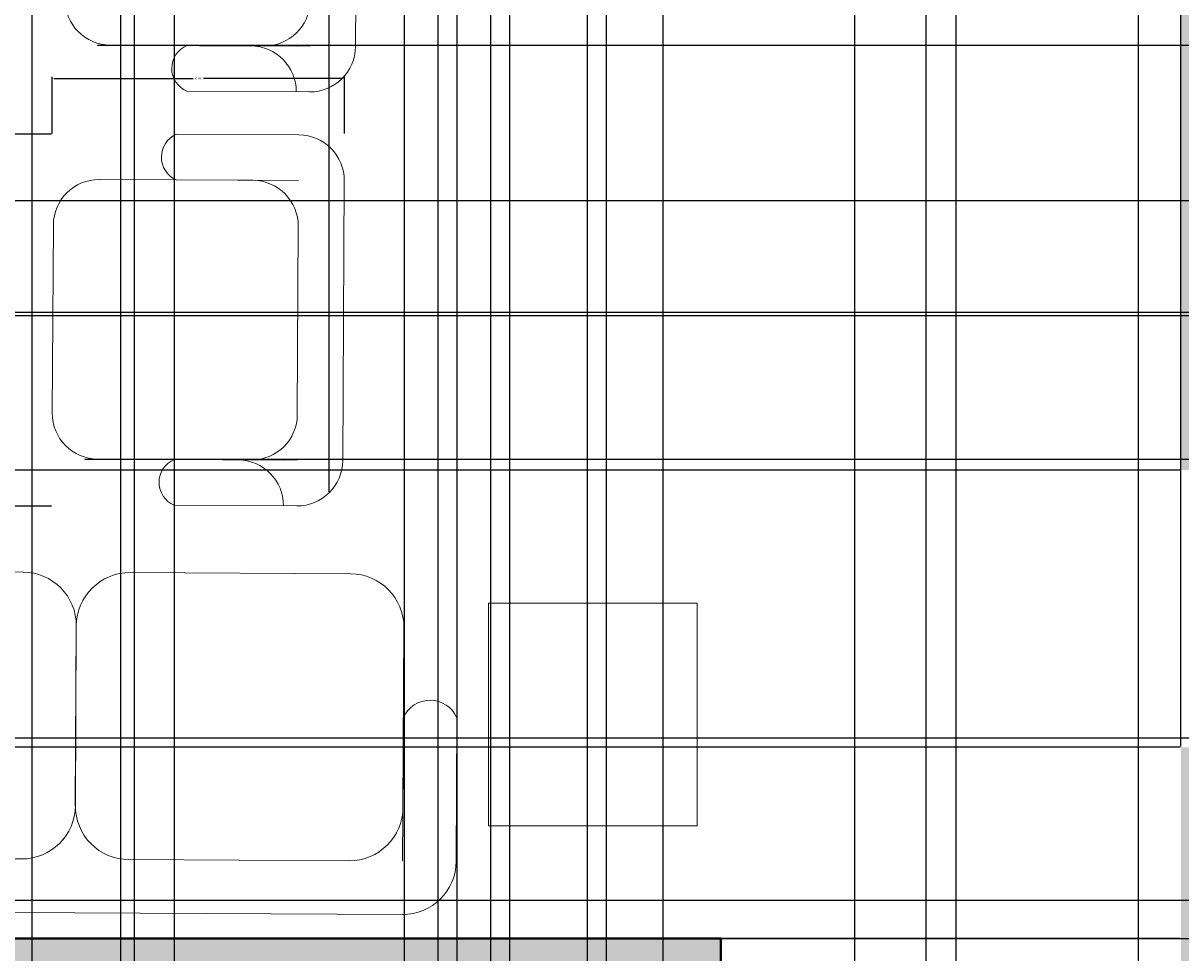
# Model space of a CAD drawing. Units: inches. Extents: x 818 to 1898, y 976 to 2364.
# Tile 36 of 96: x 1391 to 1512, y 1695 to 1792. Entities that reach past the tile are written whole.
import ezdxf

# ---------------------------------------------------------------- set-up
doc = ezdxf.new("R2010")
doc.units = ezdxf.units.IN
doc.header["$LTSCALE"] = 5
doc.header["$MEASUREMENT"] = 0
for name, color, linetype, lineweight in [('A-ANNO-DIMS', 2, 'Continuous', 18), ('A-FURN', 8, 'Continuous', 18), ('A-WALL', 7, 'Continuous', 40)]:
    doc.layers.add(name, color=color, linetype=linetype, lineweight=lineweight)
doc.layers.add('A-WALL-PATT', color=251, linetype='Continuous', lineweight=13, true_color=0x636466)
doc.styles.get("Standard").update_dxf_attribs({"font": 'arial.ttf'})
doc.dimstyles.get("Standard").update_dxf_attribs({"dimtxt": 0.18, "dimasz": 0.18, "dimexe": 0.18, "dimexo": 0.0625, "dimgap": 0.09, "dimtad": 0, "dimtih": 1, "dimtoh": 1, "dimdec": 4, "dimzin": 0, "dimdsep": 46, "dimtxsty": 'Standard', "dimcen": 0.09, "dimadec": 0, "dimazin": 0, "dimtfac": 1, "dimtdec": 4, "dimtofl": 0, "dimtmove": 0, "dimatfit": 3, "dimfxl": 1, "dimtolj": 1, "dimtzin": 0, "dimarcsym": 0})

# ---------------------------------------------------------------- blocks, each defined once
blk = doc.blocks.new('SOFA-3-SEAT')
for p, q in [((39.87, 35.86), (5.7, 36.05)), ((74.05, 35.68), (39.88, 35.86)), ((108.23, 35.49), (74.06, 35.68)), ((0, 15.52), (0.08, 30.49)), ((5.59, 15.49), (5.67, 30.46)), ((34.25, 30.31), (11.25, 30.43)), ((68.34, 30.12), (45.43, 30.24)), ((102.62, 29.94), (79.51, 30.06)), ((108.12, 14.94), (108.2, 29.9)), ((113.71, 14.91), (113.79, 29.87)), ((5.64, 24.87), (5.54, 6.11)), ((39.71, 5.93), (39.81, 24.69)), ((39.82, 24.69), (39.72, 5.93)), ((73.9, 5.71), (73.9, 24.47)), ((108.07, 5.56), (108.17, 24.32)), ((11.09, 0.49), (34.09, 0.37)), ((45.27, 0.31), (68.27, 0.19)), ((79.45, 0.12), (102.45, 0))]:
    blk.add_line(p, q)
for centre, radius, start, end in [((5.67, 30.46), 5.59, 89.6898, 179.6898), ((108.2, 29.9), 5.59, 359.6898, 89.6898), ((11.22, 24.84), 5.59, 89.6898, 179.6898), ((34.22, 24.72), 5.59, 359.6898, 89.6898), ((45.4, 24.66), 5.59, 89.6898, 179.6898), ((68.31, 24.53), 5.59, 0, 89.6898), ((79.48, 24.47), 5.59, 89.6898, 180), ((102.59, 24.35), 5.59, 359.6898, 89.6898), ((2.8, 16.75), 3.06, 203.7099, 335.6698), ((110.92, 16.05), 3.01, 201.7034, 337.6762), ((11.12, 6.08), 5.59, 179.6898, 269.6898), ((34.12, 5.96), 5.59, 269.6898, 359.6898), ((45.3, 5.9), 5.59, 179.6898, 269.6898), ((68.3, 5.77), 5.59, 269.6898, 359.6898), ((79.48, 5.71), 5.59, 179.6898, 269.6898), ((102.48, 5.59), 5.59, 269.6898, 359.6898)]:
    blk.add_arc(centre, radius, start, end)
blk = doc.blocks.new('CHAIR-LOUNGE')
for p, q in [((12.94, 38.78), (25.71, 38.71)), ((20.92, 33.97), (4.9, 34.05)), ((12.91, 34.01), (25.69, 33.94)), ((30.3, 4.74), (30.46, 33.92)), ((0.11, 29.31), (0, 9.68)), ((25.56, 9.54), (25.66, 29.17)), ((19.37, 4.79), (3.35, 4.88)), ((4.74, 4.88), (20.76, 4.79)), ((11.36, 4.84), (24.14, 4.77)), ((12.75, 4.84), (25.53, 4.77)), ((12.73, 0.07), (25.5, 0))]:
    blk.add_line(p, q)
for centre, radius, start, end in [((13.99, 36.39), 2.61, 113.7099, 245.6698), ((25.69, 33.94), 4.77, 359.6898, 89.6898), ((4.88, 29.29), 4.77, 89.6898, 179.6898), ((20.89, 29.2), 4.77, 359.6898, 89.6898), ((4.77, 9.65), 4.77, 179.6898, 269.6898), ((20.79, 9.56), 4.77, 269.6898, 359.6898), ((13.7, 2.45), 2.57, 111.7034, 247.6762), ((19.35, 0.03), 4.77, 359.6898, 89.6898), ((25.53, 4.77), 4.77, 269.6898, 359.6898)]:
    blk.add_arc(centre, radius, start, end)
blk = doc.blocks.new('*D50')
at = {"layer": 'A-ANNO-DIMS', "color": 0, "lineweight": -2, "ltscale": 5, "transparency": 16777216}
for p, q in [((1393.92, 1780.01), (1387.99, 1780.01)), ((1388.17, 1779.83), (1388.17, 1760.8)), ((1388.17, 1741.4), (1388.17, 1760.43)), ((1393.92, 1741.22), (1387.99, 1741.22))]:
    blk.add_line(p, q, dxfattribs=at)
at = {"layer": 'A-ANNO-DIMS', "color": 0, "ltscale": 5, "transparency": 16777216}
for points in [[(1388.14, 1779.83), (1388.2, 1779.83), (1388.17, 1780.01)], [(1388.14, 1741.4), (1388.2, 1741.4), (1388.17, 1741.22)]]:
    blk.add_solid(points, dxfattribs=at)
at = {"layer": 'Defpoints', "color": 0, "ltscale": 5, "transparency": 16777216}
for p in [(1388.17, 1780.01), (1393.99, 1780.01), (1393.99, 1741.22)]:
    blk.add_point(p, dxfattribs=at)
at = {"layer": 'A-ANNO-DIMS', "color": 0, "ltscale": 5, "transparency": 16777216, "insert": (1388.17, 1760.62), "char_height": 0.18, "attachment_point": 5}
blk.add_mtext('\\A1;CHAIR 39 TYP.', dxfattribs=at)
blk = doc.blocks.new('*D51')
at = {"layer": 'A-ANNO-DIMS', "color": 0, "lineweight": -2, "ltscale": 5, "transparency": 16777216}
for p, q in [((1393.99, 1780.08), (1393.99, 1786.01)), ((1394.17, 1785.83), (1408.7, 1785.83)), ((1424.28, 1785.83), (1409.75, 1785.83)), ((1424.46, 1780.08), (1424.46, 1786.01))]:
    blk.add_line(p, q, dxfattribs=at)
at = {"layer": 'A-ANNO-DIMS', "color": 0, "ltscale": 5, "transparency": 16777216}
for points in [[(1394.17, 1785.86), (1394.17, 1785.8), (1393.99, 1785.83)], [(1424.28, 1785.86), (1424.28, 1785.8), (1424.46, 1785.83)]]:
    blk.add_solid(points, dxfattribs=at)
at = {"layer": 'Defpoints', "color": 0, "ltscale": 5, "transparency": 16777216}
for p in [(1424.46, 1785.83), (1393.99, 1780.01), (1424.46, 1780.01)]:
    blk.add_point(p, dxfattribs=at)
at = {"layer": 'A-ANNO-DIMS', "color": 0, "ltscale": 5, "transparency": 16777216, "insert": (1409.22, 1785.83), "char_height": 0.18, "attachment_point": 5}
blk.add_mtext('\\A1;30 TYP.', dxfattribs=at)
blk = doc.blocks.new('*D61')
at = {"layer": 'A-ANNO-DIMS', "color": 0, "lineweight": -2, "ltscale": 5, "transparency": 16777216}
for p, q in [((1071.73, 1203.03), (1071.73, 2363.87)), ((1071.91, 2363.69), (1250.94, 2363.69)), ((1430.55, 2363.69), (1251.51, 2363.69)), ((1430.73, 1203.03), (1430.73, 2363.87))]:
    blk.add_line(p, q, dxfattribs=at)
at = {"layer": 'A-ANNO-DIMS', "color": 0, "ltscale": 5, "transparency": 16777216}
for points in [[(1071.91, 2363.72), (1071.91, 2363.66), (1071.73, 2363.69)], [(1430.55, 2363.72), (1430.55, 2363.66), (1430.73, 2363.69)]]:
    blk.add_solid(points, dxfattribs=at)
at = {"layer": 'Defpoints', "color": 0, "ltscale": 5, "transparency": 16777216}
for p in [(1430.73, 2363.69), (1071.73, 1202.96), (1430.73, 1202.96)]:
    blk.add_point(p, dxfattribs=at)
at = {"layer": 'A-ANNO-DIMS', "color": 0, "ltscale": 5, "transparency": 16777216, "insert": (1251.23, 2363.69), "char_height": 0.18, "attachment_point": 5}
blk.add_mtext('\\A1;359', dxfattribs=at)
blk = doc.blocks.new('*D64')
at = {"layer": 'A-ANNO-DIMS', "color": 0, "lineweight": -2, "ltscale": 5, "transparency": 16777216}
for p, q in [((1197.73, 1501.14), (1197.73, 2363.87)), ((1197.91, 2363.69), (1313.93, 2363.69)), ((1430.55, 2363.69), (1314.52, 2363.69)), ((1430.73, 1501.14), (1430.73, 2363.87))]:
    blk.add_line(p, q, dxfattribs=at)
at = {"layer": 'A-ANNO-DIMS', "color": 0, "ltscale": 5, "transparency": 16777216}
for points in [[(1197.91, 2363.72), (1197.91, 2363.66), (1197.73, 2363.69)], [(1430.55, 2363.72), (1430.55, 2363.66), (1430.73, 2363.69)]]:
    blk.add_solid(points, dxfattribs=at)
at = {"layer": 'Defpoints', "color": 0, "ltscale": 5, "transparency": 16777216}
for p in [(1430.73, 2363.69), (1197.73, 1501.08), (1430.73, 1501.08)]:
    blk.add_point(p, dxfattribs=at)
at = {"layer": 'A-ANNO-DIMS', "color": 0, "ltscale": 5, "transparency": 16777216, "insert": (1314.23, 2363.69), "char_height": 0.18, "attachment_point": 5}
blk.add_mtext('\\A1;233', dxfattribs=at)
blk = doc.blocks.new('*D85')
at = {"layer": 'A-ANNO-DIMS', "color": 0, "lineweight": -2, "ltscale": 5, "transparency": 16777216}
for p, q in [((1258.79, 2053.08), (1897.92, 2053.08)), ((1897.74, 2052.9), (1897.74, 1876.76)), ((1897.74, 1700.26), (1897.74, 1876.4)), ((1258.79, 1700.08), (1897.92, 1700.08))]:
    blk.add_line(p, q, dxfattribs=at)
at = {"layer": 'A-ANNO-DIMS', "color": 0, "ltscale": 5, "transparency": 16777216}
for points in [[(1897.71, 2052.9), (1897.77, 2052.9), (1897.74, 2053.08)], [(1897.71, 1700.26), (1897.77, 1700.26), (1897.74, 1700.08)]]:
    blk.add_solid(points, dxfattribs=at)
at = {"layer": 'Defpoints', "color": 0, "ltscale": 5, "transparency": 16777216}
for p in [(1258.73, 2053.08), (1897.74, 2053.08), (1258.73, 1700.08)]:
    blk.add_point(p, dxfattribs=at)
at = {"layer": 'A-ANNO-DIMS', "color": 0, "ltscale": 5, "transparency": 16777216, "insert": (1897.74, 1876.58), "char_height": 0.18, "attachment_point": 5}
blk.add_mtext('\\A1;353', dxfattribs=at)
blk = doc.blocks.new('*D98')
at = {"layer": 'A-ANNO-DIMS', "color": 0, "lineweight": -2, "ltscale": 5, "transparency": 16777216}
for p, q in [((1338.54, 1071.12), (1338.54, 2363.87)), ((1338.72, 2363.69), (1364.81, 2363.69)), ((1391.7, 2363.69), (1365.6, 2363.69)), ((1391.88, 1071.12), (1391.88, 2363.87))]:
    blk.add_line(p, q, dxfattribs=at)
at = {"layer": 'A-ANNO-DIMS', "color": 0, "ltscale": 5, "transparency": 16777216}
for points in [[(1338.72, 2363.72), (1338.72, 2363.66), (1338.54, 2363.69)], [(1391.7, 2363.72), (1391.7, 2363.66), (1391.88, 2363.69)]]:
    blk.add_solid(points, dxfattribs=at)
at = {"layer": 'Defpoints', "color": 0, "ltscale": 5, "transparency": 16777216}
for p in [(1391.88, 2363.69), (1338.54, 1071.06), (1391.88, 1071.06)]:
    blk.add_point(p, dxfattribs=at)
at = {"layer": 'A-ANNO-DIMS', "color": 0, "ltscale": 5, "transparency": 16777216, "insert": (1365.21, 2363.69), "char_height": 0.18, "attachment_point": 5}
blk.add_mtext('\\A1;53.33', dxfattribs=at)
blk = doc.blocks.new('*D99')
at = {"layer": 'A-ANNO-DIMS', "color": 0, "lineweight": -2, "ltscale": 5, "transparency": 16777216}
for p, q in [((1391.88, 1071.12), (1391.88, 2363.87)), ((1392.06, 2363.69), (1420.45, 2363.69)), ((1449.64, 2363.69), (1421.24, 2363.69)), ((1449.82, 1071.12), (1449.82, 2363.87))]:
    blk.add_line(p, q, dxfattribs=at)
at = {"layer": 'A-ANNO-DIMS', "color": 0, "ltscale": 5, "transparency": 16777216}
for points in [[(1392.06, 2363.72), (1392.06, 2363.66), (1391.88, 2363.69)], [(1449.64, 2363.72), (1449.64, 2363.66), (1449.82, 2363.69)]]:
    blk.add_solid(points, dxfattribs=at)
at = {"layer": 'Defpoints', "color": 0, "ltscale": 5, "transparency": 16777216}
for p in [(1449.82, 2363.69), (1391.88, 1071.06), (1449.82, 1071.06)]:
    blk.add_point(p, dxfattribs=at)
at = {"layer": 'A-ANNO-DIMS', "color": 0, "ltscale": 5, "transparency": 16777216, "insert": (1420.85, 2363.69), "char_height": 0.18, "attachment_point": 5}
blk.add_mtext('\\A1;57.94', dxfattribs=at)
blk = doc.blocks.new('*D100')
at = {"layer": 'A-ANNO-DIMS', "color": 0, "lineweight": -2, "ltscale": 5, "transparency": 16777216}
for p, q in [((1449.82, 1071.12), (1449.82, 2363.87)), ((1450, 2363.69), (1478.17, 2363.69)), ((1507.12, 2363.69), (1478.95, 2363.69)), ((1507.3, 1071.12), (1507.3, 2363.87))]:
    blk.add_line(p, q, dxfattribs=at)
at = {"layer": 'A-ANNO-DIMS', "color": 0, "ltscale": 5, "transparency": 16777216}
for points in [[(1450, 2363.72), (1450, 2363.66), (1449.82, 2363.69)], [(1507.12, 2363.72), (1507.12, 2363.66), (1507.3, 2363.69)]]:
    blk.add_solid(points, dxfattribs=at)
at = {"layer": 'Defpoints', "color": 0, "ltscale": 5, "transparency": 16777216}
for p in [(1507.3, 2363.69), (1449.82, 1071.06), (1507.3, 1071.06)]:
    blk.add_point(p, dxfattribs=at)
at = {"layer": 'A-ANNO-DIMS', "color": 0, "ltscale": 5, "transparency": 16777216, "insert": (1478.56, 2363.69), "char_height": 0.18, "attachment_point": 5}
blk.add_mtext('\\A1;57.48', dxfattribs=at)
blk = doc.blocks.new('*D101')
at = {"layer": 'A-ANNO-DIMS', "color": 0, "lineweight": -2, "ltscale": 5, "transparency": 16777216}
for p, q in [((1507.3, 1071.12), (1507.3, 2363.87)), ((1507.48, 2363.69), (1536, 2363.69)), ((1565.3, 2363.69), (1536.78, 2363.69)), ((1565.48, 1071.12), (1565.48, 2363.87))]:
    blk.add_line(p, q, dxfattribs=at)
at = {"layer": 'A-ANNO-DIMS', "color": 0, "ltscale": 5, "transparency": 16777216}
for points in [[(1507.48, 2363.72), (1507.48, 2363.66), (1507.3, 2363.69)], [(1565.3, 2363.72), (1565.3, 2363.66), (1565.48, 2363.69)]]:
    blk.add_solid(points, dxfattribs=at)
at = {"layer": 'Defpoints', "color": 0, "ltscale": 5, "transparency": 16777216}
for p in [(1565.48, 2363.69), (1507.3, 1071.06), (1565.48, 1071.06)]:
    blk.add_point(p, dxfattribs=at)
at = {"layer": 'A-ANNO-DIMS', "color": 0, "ltscale": 5, "transparency": 16777216, "insert": (1536.39, 2363.69), "char_height": 0.18, "attachment_point": 5}
blk.add_mtext('\\A1;58.19', dxfattribs=at)
blk = doc.blocks.new('*D119')
at = {"layer": 'A-ANNO-DIMS', "color": 0, "lineweight": -2, "ltscale": 5, "transparency": 16777216}
for p, q in [((1766.29, 1716.99), (818.03, 1716.99)), ((818.21, 1716.81), (818.21, 1672.43)), ((818.21, 1627.69), (818.21, 1672.06)), ((1766.29, 1627.51), (818.03, 1627.51))]:
    blk.add_line(p, q, dxfattribs=at)
at = {"layer": 'A-ANNO-DIMS', "color": 0, "ltscale": 5, "transparency": 16777216}
for points in [[(818.18, 1716.81), (818.24, 1716.81), (818.21, 1716.99)], [(818.18, 1627.69), (818.24, 1627.69), (818.21, 1627.51)]]:
    blk.add_solid(points, dxfattribs=at)
at = {"layer": 'Defpoints', "color": 0, "ltscale": 5, "transparency": 16777216}
for p in [(818.21, 1716.99), (1766.35, 1716.99), (1766.35, 1627.51)]:
    blk.add_point(p, dxfattribs=at)
at = {"layer": 'A-ANNO-DIMS', "color": 0, "ltscale": 5, "transparency": 16777216, "insert": (818.21, 1672.25), "char_height": 0.18, "attachment_point": 5}
blk.add_mtext('\\A1;89.48', dxfattribs=at)
blk = doc.blocks.new('*D120')
at = {"layer": 'A-ANNO-DIMS', "color": 0, "lineweight": -2, "ltscale": 5, "transparency": 16777216}
for p, q in [((1766.29, 1797.72), (818.03, 1797.72)), ((818.21, 1797.54), (818.21, 1757.53)), ((818.21, 1717.17), (818.21, 1757.17)), ((1766.29, 1716.99), (818.03, 1716.99))]:
    blk.add_line(p, q, dxfattribs=at)
at = {"layer": 'A-ANNO-DIMS', "color": 0, "ltscale": 5, "transparency": 16777216}
for points in [[(818.18, 1797.54), (818.24, 1797.54), (818.21, 1797.72)], [(818.18, 1717.17), (818.24, 1717.17), (818.21, 1716.99)]]:
    blk.add_solid(points, dxfattribs=at)
at = {"layer": 'Defpoints', "color": 0, "ltscale": 5, "transparency": 16777216}
for p in [(818.21, 1797.72), (1766.35, 1797.72), (1766.35, 1716.99)]:
    blk.add_point(p, dxfattribs=at)
at = {"layer": 'A-ANNO-DIMS', "color": 0, "ltscale": 5, "transparency": 16777216, "insert": (818.21, 1757.35), "char_height": 0.18, "attachment_point": 5}
blk.add_mtext('\\A1;80.73', dxfattribs=at)
blk = doc.blocks.new('*D166')
at = {"layer": 'A-ANNO-DIMS', "color": 0, "lineweight": -2, "ltscale": 5, "transparency": 16777216}
for p, q in [((1401.15, 1510.14), (1401.15, 2363.87)), ((1401.33, 2363.69), (1415.54, 2363.69)), ((1430.55, 2363.69), (1416.33, 2363.69)), ((1430.73, 1510.14), (1430.73, 2363.87))]:
    blk.add_line(p, q, dxfattribs=at)
at = {"layer": 'A-ANNO-DIMS', "color": 0, "ltscale": 5, "transparency": 16777216}
for points in [[(1401.33, 2363.72), (1401.33, 2363.66), (1401.15, 2363.69)], [(1430.55, 2363.72), (1430.55, 2363.66), (1430.73, 2363.69)]]:
    blk.add_solid(points, dxfattribs=at)
at = {"layer": 'Defpoints', "color": 0, "ltscale": 5, "transparency": 16777216}
for p in [(1430.73, 2363.69), (1401.15, 1510.08), (1430.73, 1510.08)]:
    blk.add_point(p, dxfattribs=at)
at = {"layer": 'A-ANNO-DIMS', "color": 0, "ltscale": 5, "transparency": 16777216, "insert": (1415.94, 2363.69), "char_height": 0.18, "attachment_point": 5}
blk.add_mtext('\\A1;29.58', dxfattribs=at)
blk = doc.blocks.new('*D169')
at = {"layer": 'A-ANNO-DIMS', "color": 0, "lineweight": -2, "ltscale": 5, "transparency": 16777216}
for p, q in [((1441.73, 1600.14), (1441.73, 2363.87)), ((1441.91, 2363.69), (1459.51, 2363.69)), ((1477.55, 2363.69), (1459.94, 2363.69)), ((1477.73, 1600.14), (1477.73, 2363.87))]:
    blk.add_line(p, q, dxfattribs=at)
at = {"layer": 'A-ANNO-DIMS', "color": 0, "ltscale": 5, "transparency": 16777216}
for points in [[(1441.91, 2363.72), (1441.91, 2363.66), (1441.73, 2363.69)], [(1477.55, 2363.72), (1477.55, 2363.66), (1477.73, 2363.69)]]:
    blk.add_solid(points, dxfattribs=at)
at = {"layer": 'Defpoints', "color": 0, "ltscale": 5, "transparency": 16777216}
for p in [(1477.73, 2363.69), (1441.73, 1600.08), (1477.73, 1600.08)]:
    blk.add_point(p, dxfattribs=at)
at = {"layer": 'A-ANNO-DIMS', "color": 0, "ltscale": 5, "transparency": 16777216, "insert": (1459.73, 2363.69), "char_height": 0.18, "attachment_point": 5}
blk.add_mtext('\\A1;36', dxfattribs=at)
blk = doc.blocks.new('*D191')
at = {"layer": 'A-ANNO-DIMS', "color": 0, "lineweight": -2, "ltscale": 5, "transparency": 16777216}
for p, q in [((1434.23, 1409.11), (1434.23, 2363.87)), ((1434.41, 2363.69), (1435.08, 2363.69)), ((1436.05, 2363.69), (1435.37, 2363.69)), ((1436.23, 1409.11), (1436.23, 2363.87))]:
    blk.add_line(p, q, dxfattribs=at)
at = {"layer": 'A-ANNO-DIMS', "color": 0, "ltscale": 5, "transparency": 16777216}
for points in [[(1434.41, 2363.72), (1434.41, 2363.66), (1434.23, 2363.69)], [(1436.05, 2363.72), (1436.05, 2363.66), (1436.23, 2363.69)]]:
    blk.add_solid(points, dxfattribs=at)
at = {"layer": 'Defpoints', "color": 0, "ltscale": 5, "transparency": 16777216}
for p in [(1436.23, 2363.69), (1434.23, 1409.05), (1436.23, 1409.05)]:
    blk.add_point(p, dxfattribs=at)
at = {"layer": 'A-ANNO-DIMS', "color": 0, "ltscale": 5, "transparency": 16777216, "insert": (1435.23, 2363.69), "char_height": 0.18, "attachment_point": 5}
blk.add_mtext('\\A1;2', dxfattribs=at)
blk = doc.blocks.new('*D196')
at = {"layer": 'A-ANNO-DIMS', "color": 0, "lineweight": -2, "ltscale": 5, "transparency": 16777216}
for p, q in [((1439.73, 1526.73), (1439.73, 2363.87)), ((1439.91, 2363.69), (1448.51, 2363.69)), ((1457.55, 2363.69), (1448.94, 2363.69)), ((1457.73, 1526.73), (1457.73, 2363.87))]:
    blk.add_line(p, q, dxfattribs=at)
at = {"layer": 'A-ANNO-DIMS', "color": 0, "ltscale": 5, "transparency": 16777216}
for points in [[(1439.91, 2363.72), (1439.91, 2363.66), (1439.73, 2363.69)], [(1457.55, 2363.72), (1457.55, 2363.66), (1457.73, 2363.69)]]:
    blk.add_solid(points, dxfattribs=at)
at = {"layer": 'Defpoints', "color": 0, "ltscale": 5, "transparency": 16777216}
for p in [(1457.73, 2363.69), (1439.73, 1526.67), (1457.73, 1526.67)]:
    blk.add_point(p, dxfattribs=at)
at = {"layer": 'A-ANNO-DIMS', "color": 0, "ltscale": 5, "transparency": 16777216, "insert": (1448.73, 2363.69), "char_height": 0.18, "attachment_point": 5}
blk.add_mtext('\\A1;18', dxfattribs=at)
blk = doc.blocks.new('*D215')
at = {"layer": 'A-ANNO-DIMS', "color": 0, "lineweight": -2, "ltscale": 5, "transparency": 16777216}
for p, q in [((1590.66, 1876.08), (818.03, 1876.08)), ((818.21, 1875.9), (818.21, 1781.76)), ((818.21, 1687.26), (818.21, 1781.4)), ((1511.66, 1687.08), (818.03, 1687.08))]:
    blk.add_line(p, q, dxfattribs=at)
at = {"layer": 'A-ANNO-DIMS', "color": 0, "ltscale": 5, "transparency": 16777216}
for points in [[(818.18, 1875.9), (818.24, 1875.9), (818.21, 1876.08)], [(818.18, 1687.26), (818.24, 1687.26), (818.21, 1687.08)]]:
    blk.add_solid(points, dxfattribs=at)
at = {"layer": 'Defpoints', "color": 0, "ltscale": 5, "transparency": 16777216}
for p in [(818.21, 1876.08), (1590.73, 1876.08), (1511.73, 1687.08)]:
    blk.add_point(p, dxfattribs=at)
at = {"layer": 'A-ANNO-DIMS', "color": 0, "ltscale": 5, "transparency": 16777216, "insert": (818.21, 1781.58), "char_height": 0.18, "attachment_point": 5}
blk.add_mtext('\\A1;189', dxfattribs=at)
blk = doc.blocks.new('*D220')
at = {"layer": 'A-ANNO-DIMS', "color": 0, "lineweight": -2, "ltscale": 5, "transparency": 16777216}
for p, q in [((1520.66, 1773.08), (818.03, 1773.08)), ((818.21, 1772.9), (818.21, 1767.26)), ((818.21, 1761.26), (818.21, 1766.9)), ((1520.66, 1761.08), (818.03, 1761.08))]:
    blk.add_line(p, q, dxfattribs=at)
at = {"layer": 'A-ANNO-DIMS', "color": 0, "ltscale": 5, "transparency": 16777216}
for points in [[(818.18, 1772.9), (818.24, 1772.9), (818.21, 1773.08)], [(818.18, 1761.26), (818.24, 1761.26), (818.21, 1761.08)]]:
    blk.add_solid(points, dxfattribs=at)
at = {"layer": 'Defpoints', "color": 0, "ltscale": 5, "transparency": 16777216}
for p in [(818.21, 1773.08), (1520.73, 1773.08), (1520.73, 1761.08)]:
    blk.add_point(p, dxfattribs=at)
at = {"layer": 'A-ANNO-DIMS', "color": 0, "ltscale": 5, "transparency": 16777216, "insert": (818.21, 1767.08), "char_height": 0.18, "attachment_point": 5}
blk.add_mtext('\\A1;12', dxfattribs=at)
blk = doc.blocks.new('*D222')
at = {"layer": 'A-ANNO-DIMS', "color": 0, "lineweight": -2, "ltscale": 5, "transparency": 16777216}
for p, q in [((1511.66, 1744.97), (818.03, 1744.97)), ((818.21, 1744.79), (818.21, 1730.69)), ((818.21, 1716.23), (818.21, 1730.33)), ((1511.66, 1716.05), (818.03, 1716.05))]:
    blk.add_line(p, q, dxfattribs=at)
at = {"layer": 'A-ANNO-DIMS', "color": 0, "ltscale": 5, "transparency": 16777216}
for points in [[(818.18, 1744.79), (818.24, 1744.79), (818.21, 1744.97)], [(818.18, 1716.23), (818.24, 1716.23), (818.21, 1716.05)]]:
    blk.add_solid(points, dxfattribs=at)
at = {"layer": 'Defpoints', "color": 0, "ltscale": 5, "transparency": 16777216}
for p in [(818.21, 1744.97), (1511.73, 1744.97), (1511.73, 1716.05)]:
    blk.add_point(p, dxfattribs=at)
at = {"layer": 'A-ANNO-DIMS', "color": 0, "ltscale": 5, "transparency": 16777216, "insert": (818.21, 1730.51), "char_height": 0.18, "attachment_point": 5}
blk.add_mtext('\\A1;28.926', dxfattribs=at)
blk = doc.blocks.new('*D223')
at = {"layer": 'A-ANNO-DIMS', "color": 0, "lineweight": -2, "ltscale": 5, "transparency": 16777216}
for p, q in [((1511.66, 1716.05), (818.03, 1716.05)), ((818.21, 1715.87), (818.21, 1706.24)), ((818.21, 1696.26), (818.21, 1705.88)), ((1511.66, 1696.08), (818.03, 1696.08))]:
    blk.add_line(p, q, dxfattribs=at)
at = {"layer": 'A-ANNO-DIMS', "color": 0, "ltscale": 5, "transparency": 16777216}
for points in [[(818.18, 1715.87), (818.24, 1715.87), (818.21, 1716.05)], [(818.18, 1696.26), (818.24, 1696.26), (818.21, 1696.08)]]:
    blk.add_solid(points, dxfattribs=at)
at = {"layer": 'Defpoints', "color": 0, "ltscale": 5, "transparency": 16777216}
for p in [(818.21, 1716.05), (1511.73, 1716.05), (1511.73, 1696.08)]:
    blk.add_point(p, dxfattribs=at)
at = {"layer": 'A-ANNO-DIMS', "color": 0, "ltscale": 5, "transparency": 16777216, "insert": (818.21, 1706.06), "char_height": 0.18, "attachment_point": 5}
blk.add_mtext('\\A1;19.967', dxfattribs=at)
blk = doc.blocks.new('*D231')
at = {"layer": 'A-ANNO-DIMS', "color": 0, "lineweight": -2, "ltscale": 5, "transparency": 16777216}
for p, q in [((1303.93, 1952.98), (1303.93, 975.66)), ((1402.52, 1952.98), (1402.52, 975.66)), ((1304.11, 975.84), (1352.83, 975.84)), ((1402.34, 975.84), (1353.62, 975.84))]:
    blk.add_line(p, q, dxfattribs=at)
at = {"layer": 'A-ANNO-DIMS', "color": 0, "ltscale": 5, "transparency": 16777216}
for points in [[(1304.11, 975.87), (1304.11, 975.81), (1303.93, 975.84)], [(1402.34, 975.87), (1402.34, 975.81), (1402.52, 975.84)]]:
    blk.add_solid(points, dxfattribs=at)
at = {"layer": 'Defpoints', "color": 0, "ltscale": 5, "transparency": 16777216}
for p in [(1303.93, 1953.04), (1402.52, 1953.04), (1402.52, 975.84)]:
    blk.add_point(p, dxfattribs=at)
at = {"layer": 'A-ANNO-DIMS', "color": 0, "ltscale": 5, "transparency": 16777216, "insert": (1353.22, 975.84), "char_height": 0.18, "attachment_point": 5}
blk.add_mtext('\\A1;98.59', dxfattribs=at)
blk = doc.blocks.new('*D242')
at = {"layer": 'A-ANNO-DIMS', "color": 0, "lineweight": -2, "ltscale": 5, "transparency": 16777216}
for p, q in [((1488.26, 1948.6), (1488.26, 975.66)), ((1513.23, 1948.6), (1513.23, 975.66)), ((1488.44, 975.84), (1500.35, 975.84)), ((1513.05, 975.84), (1501.14, 975.84))]:
    blk.add_line(p, q, dxfattribs=at)
at = {"layer": 'A-ANNO-DIMS', "color": 0, "ltscale": 5, "transparency": 16777216}
for points in [[(1488.44, 975.87), (1488.44, 975.81), (1488.26, 975.84)], [(1513.05, 975.87), (1513.05, 975.81), (1513.23, 975.84)]]:
    blk.add_solid(points, dxfattribs=at)
at = {"layer": 'Defpoints', "color": 0, "ltscale": 5, "transparency": 16777216}
for p in [(1488.26, 1948.66), (1513.23, 1948.66), (1513.23, 975.84)]:
    blk.add_point(p, dxfattribs=at)
at = {"layer": 'A-ANNO-DIMS', "color": 0, "ltscale": 5, "transparency": 16777216, "insert": (1500.74, 975.84), "char_height": 0.18, "attachment_point": 5}
blk.add_mtext('\\A1;24.97', dxfattribs=at)
blk = doc.blocks.new('*D243')
at = {"layer": 'A-ANNO-DIMS', "color": 0, "lineweight": -2, "ltscale": 5, "transparency": 16777216}
for p, q in [((1451.77, 2020.02), (1451.77, 975.66)), ((1590.73, 2020.02), (1590.73, 975.66)), ((1451.95, 975.84), (1520.79, 975.84)), ((1590.55, 975.84), (1521.7, 975.84))]:
    blk.add_line(p, q, dxfattribs=at)
at = {"layer": 'A-ANNO-DIMS', "color": 0, "ltscale": 5, "transparency": 16777216}
for points in [[(1451.95, 975.87), (1451.95, 975.81), (1451.77, 975.84)], [(1590.55, 975.87), (1590.55, 975.81), (1590.73, 975.84)]]:
    blk.add_solid(points, dxfattribs=at)
at = {"layer": 'Defpoints', "color": 0, "ltscale": 5, "transparency": 16777216}
for p in [(1451.77, 2020.08), (1590.73, 2020.08), (1590.73, 975.84)]:
    blk.add_point(p, dxfattribs=at)
at = {"layer": 'A-ANNO-DIMS', "color": 0, "ltscale": 5, "transparency": 16777216, "insert": (1521.25, 975.84), "char_height": 0.18, "attachment_point": 5}
blk.add_mtext('\\A1;138.96', dxfattribs=at)
blk = doc.blocks.new('*D253')
at = {"layer": 'A-ANNO-DIMS', "color": 0, "lineweight": -2, "ltscale": 5, "transparency": 16777216}
for p, q in [((1485.12, 2053.02), (1485.12, 975.66)), ((1538.52, 2053.02), (1538.52, 975.66)), ((1485.3, 975.84), (1511.42, 975.84)), ((1538.34, 975.84), (1512.21, 975.84))]:
    blk.add_line(p, q, dxfattribs=at)
at = {"layer": 'A-ANNO-DIMS', "color": 0, "ltscale": 5, "transparency": 16777216}
for points in [[(1485.3, 975.87), (1485.3, 975.81), (1485.12, 975.84)], [(1538.34, 975.87), (1538.34, 975.81), (1538.52, 975.84)]]:
    blk.add_solid(points, dxfattribs=at)
at = {"layer": 'Defpoints', "color": 0, "ltscale": 5, "transparency": 16777216}
for p in [(1485.12, 2053.08), (1538.52, 2053.08), (1538.52, 975.84)]:
    blk.add_point(p, dxfattribs=at)
at = {"layer": 'A-ANNO-DIMS', "color": 0, "ltscale": 5, "transparency": 16777216, "insert": (1511.82, 975.84), "char_height": 0.18, "attachment_point": 5}
blk.add_mtext('\\A1;53.39', dxfattribs=at)
blk = doc.blocks.new('*D273')
at = {"layer": 'A-ANNO-DIMS', "color": 0, "lineweight": -2, "ltscale": 5, "transparency": 16777216}
for p, q in [((1406.73, 1587.48), (1406.73, 2363.87)), ((1406.91, 2363.69), (1418.51, 2363.69)), ((1430.55, 2363.69), (1418.95, 2363.69)), ((1430.73, 1587.48), (1430.73, 2363.87))]:
    blk.add_line(p, q, dxfattribs=at)
at = {"layer": 'A-ANNO-DIMS', "color": 0, "ltscale": 5, "transparency": 16777216}
for points in [[(1406.91, 2363.72), (1406.91, 2363.66), (1406.73, 2363.69)], [(1430.55, 2363.72), (1430.55, 2363.66), (1430.73, 2363.69)]]:
    blk.add_solid(points, dxfattribs=at)
at = {"layer": 'Defpoints', "color": 0, "ltscale": 5, "transparency": 16777216}
for p in [(1430.73, 2363.69), (1406.73, 1587.42), (1430.73, 1587.42)]:
    blk.add_point(p, dxfattribs=at)
at = {"layer": 'A-ANNO-DIMS', "color": 0, "ltscale": 5, "transparency": 16777216, "insert": (1418.73, 2363.69), "char_height": 0.18, "attachment_point": 5}
blk.add_mtext('\\A1;24', dxfattribs=at)
blk = doc.blocks.new('*D280')
at = {"layer": 'A-ANNO-DIMS', "color": 0, "lineweight": -2, "ltscale": 5, "transparency": 16777216}
for p, q in [((1398.73, 1789.31), (1897.92, 1789.31)), ((1897.74, 1789.13), (1897.74, 1767.89)), ((1897.74, 1746.29), (1897.74, 1767.53)), ((1397.41, 1746.11), (1897.92, 1746.11))]:
    blk.add_line(p, q, dxfattribs=at)
at = {"layer": 'A-ANNO-DIMS', "color": 0, "ltscale": 5, "transparency": 16777216}
for points in [[(1897.71, 1789.13), (1897.77, 1789.13), (1897.74, 1789.31)], [(1897.71, 1746.29), (1897.77, 1746.29), (1897.74, 1746.11)]]:
    blk.add_solid(points, dxfattribs=at)
at = {"layer": 'Defpoints', "color": 0, "ltscale": 5, "transparency": 16777216}
for p in [(1398.67, 1789.31), (1897.74, 1789.31), (1397.35, 1746.11)]:
    blk.add_point(p, dxfattribs=at)
at = {"layer": 'A-ANNO-DIMS', "color": 0, "ltscale": 5, "transparency": 16777216, "insert": (1897.74, 1767.71), "char_height": 0.18, "attachment_point": 5}
blk.add_mtext('\\A1;43.19', dxfattribs=at)
blk = doc.blocks.new('*D282')
at = {"layer": 'A-ANNO-DIMS', "color": 0, "lineweight": -2, "ltscale": 5, "transparency": 16777216}
for p, q in [((1422.08, 2081.19), (1897.92, 2081.19)), ((1897.74, 2081.01), (1897.74, 1884.32)), ((1897.74, 1687.26), (1897.74, 1883.95)), ((1463.79, 1687.08), (1897.92, 1687.08))]:
    blk.add_line(p, q, dxfattribs=at)
at = {"layer": 'A-ANNO-DIMS', "color": 0, "ltscale": 5, "transparency": 16777216}
for points in [[(1897.71, 2081.01), (1897.77, 2081.01), (1897.74, 2081.19)], [(1897.71, 1687.26), (1897.77, 1687.26), (1897.74, 1687.08)]]:
    blk.add_solid(points, dxfattribs=at)
at = {"layer": 'Defpoints', "color": 0, "ltscale": 5, "transparency": 16777216}
for p in [(1422.02, 2081.19), (1897.74, 2081.19), (1463.73, 1687.08)]:
    blk.add_point(p, dxfattribs=at)
at = {"layer": 'A-ANNO-DIMS', "color": 0, "ltscale": 5, "transparency": 16777216, "insert": (1897.74, 1884.13), "char_height": 0.18, "attachment_point": 5}
blk.add_mtext('\\A1;394.1', dxfattribs=at)
blk = doc.blocks.new('*D284')
at = {"layer": 'A-ANNO-DIMS', "color": 0, "lineweight": -2, "ltscale": 5, "transparency": 16777216}
for p, q in [((1351.66, 1761.45), (1897.92, 1761.45)), ((1897.74, 1761.27), (1897.74, 1728.95)), ((1897.74, 1696.26), (1897.74, 1728.58)), ((1267.79, 1696.08), (1897.92, 1696.08))]:
    blk.add_line(p, q, dxfattribs=at)
at = {"layer": 'A-ANNO-DIMS', "color": 0, "ltscale": 5, "transparency": 16777216}
for points in [[(1897.71, 1761.27), (1897.77, 1761.27), (1897.74, 1761.45)], [(1897.71, 1696.26), (1897.77, 1696.26), (1897.74, 1696.08)]]:
    blk.add_solid(points, dxfattribs=at)
at = {"layer": 'Defpoints', "color": 0, "ltscale": 5, "transparency": 16777216}
for p in [(1351.6, 1761.45), (1267.73, 1696.08), (1897.74, 1696.08)]:
    blk.add_point(p, dxfattribs=at)
at = {"layer": 'A-ANNO-DIMS', "color": 0, "ltscale": 5, "transparency": 16777216, "insert": (1897.74, 1728.76), "char_height": 0.18, "attachment_point": 5}
blk.add_mtext('\\A1;65.37', dxfattribs=at)
blk = doc.blocks.new('*D288')
at = {"layer": 'A-ANNO-DIMS', "color": 0, "lineweight": -2, "ltscale": 5, "transparency": 16777216}
for p, q in [((1422.88, 1742.67), (1422.88, 2363.87)), ((1423.06, 2363.69), (1466.91, 2363.69)), ((1511.55, 2363.69), (1467.69, 2363.69)), ((1511.73, 1716.11), (1511.73, 2363.87))]:
    blk.add_line(p, q, dxfattribs=at)
at = {"layer": 'A-ANNO-DIMS', "color": 0, "ltscale": 5, "transparency": 16777216}
for points in [[(1423.06, 2363.72), (1423.06, 2363.66), (1422.88, 2363.69)], [(1511.55, 2363.72), (1511.55, 2363.66), (1511.73, 2363.69)]]:
    blk.add_solid(points, dxfattribs=at)
at = {"layer": 'Defpoints', "color": 0, "ltscale": 5, "transparency": 16777216}
for p in [(1511.73, 2363.69), (1422.88, 1742.61), (1511.73, 1716.05)]:
    blk.add_point(p, dxfattribs=at)
at = {"layer": 'A-ANNO-DIMS', "color": 0, "ltscale": 5, "transparency": 16777216, "insert": (1467.3, 2363.69), "char_height": 0.18, "attachment_point": 5}
blk.add_mtext('\\A1;88.85', dxfattribs=at)

msp = doc.modelspace()

# ---------------------------------------------------------------- hatches: boundary and pattern name
at = {"layer": 'A-WALL-PATT', "ltscale": 5}
h = msp.add_hatch(color=256, dxfattribs=at)
h.dxf.hatch_style = 1
h.paths.add_polyline_path([(1267.7251, 1928.9218), (1258.7251, 1928.9218), (1258.7251, 1913.6401), (1250.3029, 1913.6401), (1250.3029, 1878.3919), (1258.7251, 1878.3919), (1258.7251, 1862.9652), (1267.7251, 1862.9652)])
h.paths.add_polyline_path([(1267.7251, 1814.9652), (1258.7251, 1814.9652), (1258.7251, 1755.3321), (1267.7251, 1755.3321)])
h.paths.add_polyline_path([(1463.7251, 1696.0782), (1267.7251, 1696.0782), (1267.7251, 1707.3321), (1258.7251, 1707.3321), (1258.7251, 1700.0782), (1251.9333, 1700.0782), (1251.9333, 1687.0782), (1463.7251, 1687.0782)])
h.paths.add_polyline_path([(1714.7252, 1717.3178), (1705.7252, 1717.3178), (1705.7252, 1696.0782), (1599.7252, 1696.0782), (1599.7252, 1790.0782), (1705.7252, 1790.0782), (1705.7252, 1785.6125), (1714.7252, 1785.6125), (1714.7252, 1827.2125), (1705.7252, 1827.2125), (1705.7252, 1802.0782), (1599.7252, 1802.0782), (1599.7252, 1867.0782), (1705.7252, 1867.0782), (1705.7252, 1857.2125), (1714.7252, 1857.2125), (1714.7252, 1930.0316), (1741.8409, 1930.0316), (1741.8409, 1935.0316), (1714.7252, 1935.0316), (1714.7252, 1957.0338), (1741.8409, 1957.0338), (1741.8409, 1962.0338), (1714.7252, 1962.0338), (1705.7252, 1962.0338), (1705.7252, 1948.0782), (1599.7252, 1948.0782), (1599.7252, 1981.0782), (1590.7251, 1981.0782), (1590.7251, 1941.0782), (1620.7252, 1941.0782), (1705.7252, 1941.0782), (1705.7252, 1876.0782), (1599.7252, 1876.0782), (1599.7252, 1911.0782), (1590.7251, 1911.0782), (1590.7251, 1876.0782), (1429.2252, 1876.0782), (1429.2252, 1867.0782), (1511.7251, 1867.0782), (1528.593, 1867.0782), (1595.7252, 1867.0782), (1595.7252, 1773.0782), (1520.7251, 1773.0782), (1520.7251, 1837.5823), (1532.593, 1837.5823), (1532.593, 1867.0782), (1528.593, 1867.0782), (1528.593, 1841.5823), (1511.7251, 1841.5823), (1511.7251, 1744.9714), (1520.7251, 1744.9714), (1520.7251, 1761.0782), (1595.7252, 1761.0782), (1595.7252, 1696.0782), (1520.7251, 1696.0782), (1520.7251, 1716.0454), (1511.7251, 1716.0454), (1511.7251, 1696.0782), (1511.7251, 1687.0782), (1714.7252, 1687.0782)])
h.paths.add_polyline_path([(1714.7252, 2053.0782), (1714.7252, 2081.1881), (1709.7252, 2081.1881), (1709.7252, 2053.0782), (1681.6446, 2053.0782), (1681.6446, 2081.1881), (1676.6446, 2081.1881), (1676.6446, 2053.0782), (1538.5155, 2053.0782), (1538.5155, 2044.0782), (1590.7251, 2044.0782), (1590.7251, 2011.0782), (1599.7252, 2011.0782), (1599.7252, 2044.0782), (1705.7252, 2044.0782), (1705.7252, 2014.5114), (1714.7252, 2014.5114)])
h.paths.add_polyline_path([(1485.1216, 2053.0782), (1422.02, 2053.0782), (1422.02, 2081.1881), (1413.02, 2081.1881), (1413.02, 2053.0782), (1399.6356, 2053.0782), (1399.6356, 2081.1881), (1390.6356, 2081.1881), (1390.6356, 2053.0782), (1388.0315, 2053.0782), (1388.0315, 2044.0782), (1416.2743, 2044.0782), (1485.1216, 2044.0782)])
h.paths.add_polyline_path([(1330.305, 2053.0782), (1258.7251, 2053.0782), (1258.7251, 2019.2871), (1267.7251, 2019.2871), (1267.7251, 2044.0782), (1330.305, 2044.0782)])
h.paths.add_polyline_path([(1258.7251, 2053.0782), (1214.6577, 2053.0782), (1214.6577, 2044.0782), (1258.7251, 2044.0782)])
h.paths.add_polyline_path([(1214.6577, 2053.0782), (1180.349, 2053.0782), (1180.349, 2044.0782), (1214.6577, 2044.0782)])
h.paths.add_polyline_path([(1714.7252, 1639.5782), (1741.8409, 1639.5782), (1741.8409, 1643.5782), (1714.7252, 1643.5782), (1714.7252, 1649.9029), (1705.7252, 1649.9029), (1705.7252, 1600.0782), (1477.7251, 1600.0782), (1477.7251, 1591.0782), (1520.7251, 1591.0782), (1616.7252, 1591.0782), (1616.7252, 1416.6857), (1622.7252, 1416.6857), (1622.7252, 1463.0782), (1624.7252, 1463.0782), (1624.7252, 1467.0782), (1622.7252, 1467.0782), (1622.7252, 1591.0782), (1705.7252, 1591.0782), (1705.7252, 1545.0782), (1714.7252, 1545.0782), (1741.8409, 1545.0782), (1741.8409, 1549.0782), (1714.7252, 1549.0782), (1714.7252, 1593.9175), (1737.8409, 1593.9175), (1737.8409, 1597.9175), (1714.7252, 1597.9175)])
h.paths.add_polyline_path([(1674.9024, 2060.7419), (1714.7045, 2060.7419), (1714.7045, 2073.1061), (1674.9024, 2073.1061)], flags=25)
h.paths.add_polyline_path([(1394.5468, 2061.6618), (1422.2344, 2061.6618), (1422.2344, 2074.0261), (1394.5468, 2074.0261)], flags=24)

# ---------------------------------------------------------------- linework, layer by layer
at = {"layer": 'A-FURN'}
msp.add_lwpolyline([(1439.4881, 1731.0947), (1461.2662, 1731.0947), (1461.2662, 1707.8508), (1439.4881, 1707.8508)], close=True, dxfattribs=at)
at = {"layer": 'A-WALL'}
for p, q in [((1267.7251, 1696.0782), (1463.7251, 1696.0782)), ((1463.7251, 1696.0782), (1463.7251, 1687.0782))]:
    msp.add_line(p, q, dxfattribs=at)

# ---------------------------------------------------------------- block references
at = {"layer": 'A-FURN'}
for p in [(1395.3178, 1784.4245), (1393.992, 1741.233)]:
    msp.add_blockref('CHAIR-LOUNGE', p, dxfattribs=at)
at = {"layer": 'A-FURN', "rotation": 180}
msp.add_blockref('SOFA-3-SEAT', (1436.207, 1734.6394), dxfattribs=at)

# ---------------------------------------------------------------- dimensions: what is measured, and where the dimension line sits
at = {"layer": 'A-ANNO-DIMS', "ltscale": 5}
for base, p1, p2, override, picture, middle in [((1430.7251, 2363.6929), (1071.7251, 1202.9642), (1430.7251, 1202.9642), {"dimdec": 0, "dimlfac": 1, "dimrnd": 0, "dimzin": 0, "dimdsep": 46, "dimlunit": 2}, '*D61', (1251.2251, 2363.6929)), ((1430.7251, 2363.6929), (1197.7251, 1501.0782), (1430.7251, 1501.0782), {"dimdec": 0, "dimlfac": 1, "dimrnd": 0, "dimzin": 0, "dimdsep": 46, "dimlunit": 2}, '*D64', (1314.2251, 2363.6929)), ((1391.8757, 2363.6929), (1338.5412, 1071.0552), (1391.8757, 1071.0552), {"dimdec": 2, "dimlfac": 1, "dimrnd": 0, "dimzin": 0, "dimdsep": 46, "dimlunit": 2}, '*D98', (1365.2084, 2363.6929)), ((1449.8196, 2363.6929), (1391.8757, 1071.0552), (1449.8196, 1071.0552), {"dimdec": 2, "dimlfac": 1, "dimrnd": 0, "dimzin": 0, "dimdsep": 46, "dimlunit": 2}, '*D99', (1420.8477, 2363.6929)), ((1430.7251, 2363.6929), (1401.1463, 1510.0782), (1430.7251, 1510.0782), {"dimdec": 2, "dimlfac": 1, "dimrnd": 0, "dimzin": 0, "dimdsep": 46, "dimlunit": 2}, '*D166', (1415.9357, 2363.6929)), ((1430.7251, 2363.6929), (1406.7251, 1587.4164), (1430.7251, 1587.4164), {"dimdec": 0, "dimlfac": 1, "dimrnd": 0, "dimzin": 0, "dimdsep": 46, "dimlunit": 2}, '*D273', (1418.7251, 2363.6929)), ((1511.7251, 2363.6929), (1422.8756, 1742.6113), (1511.7251, 1716.0454), {"dimdec": 2, "dimlfac": 1, "dimrnd": 0, "dimzin": 0, "dimdsep": 46, "dimlunit": 2}, '*D288', (1467.3004, 2363.6929)), ((1436.2251, 2363.6929), (1434.2251, 1409.0522), (1436.2251, 1409.0522), {"dimdec": 0, "dimlfac": 1, "dimrnd": 0, "dimzin": 0, "dimdsep": 46, "dimlunit": 2}, '*D191', (1435.2251, 2363.6929)), ((1457.7251, 2363.6929), (1439.7251, 1526.6712), (1457.7251, 1526.6712), {"dimdec": 0, "dimlfac": 1, "dimrnd": 0, "dimzin": 0, "dimdsep": 46, "dimlunit": 2}, '*D196', (1448.7251, 2363.6929)), ((1477.7251, 2363.6929), (1441.7251, 1600.0782), (1477.7251, 1600.0782), {"dimdec": 0, "dimlfac": 1, "dimrnd": 0, "dimzin": 0, "dimdsep": 46, "dimlunit": 2}, '*D169', (1459.7251, 2363.6929)), ((1507.2982, 2363.6929), (1449.8196, 1071.0552), (1507.2982, 1071.0552), {"dimdec": 2, "dimlfac": 1, "dimrnd": 0, "dimzin": 0, "dimdsep": 46, "dimlunit": 2}, '*D100', (1478.5589, 2363.6929)), ((1565.4835, 2363.6929), (1507.2982, 1071.0552), (1565.4835, 1071.0552), {"dimdec": 2, "dimlfac": 1, "dimrnd": 0, "dimzin": 0, "dimdsep": 46, "dimlunit": 2}, '*D101', (1536.3908, 2363.6929)), ((1538.5155, 975.8433), (1485.1216, 2053.0782), (1538.5155, 2053.0782), {"dimdec": 2, "dimlfac": 1, "dimrnd": 0, "dimzin": 0, "dimdsep": 46, "dimlunit": 2}, '*D253', (1511.8185, 975.8433)), ((1590.7251, 975.8433), (1451.7698, 2020.0782), (1590.7251, 2020.0782), {"dimdec": 2, "dimlfac": 1, "dimrnd": 0, "dimzin": 0, "dimdsep": 46, "dimlunit": 2}, '*D243', (1521.2475, 975.8433)), ((1402.518, 975.8433), (1303.9314, 1953.0408), (1402.518, 1953.0408), {"dimdec": 2, "dimlfac": 1, "dimrnd": 0, "dimzin": 0, "dimdsep": 46, "dimlunit": 2}, '*D231', (1353.2247, 975.8433)), ((1513.2306, 975.8433), (1488.2586, 1948.6602), (1513.2306, 1948.6602), {"dimdec": 2, "dimlfac": 1, "dimrnd": 0, "dimzin": 0, "dimdsep": 46, "dimlunit": 2}, '*D242', (1500.7446, 975.8433))]:
    dim = msp.add_linear_dim(base=base, p1=p1, p2=p2, dimstyle='Standard', override=override, dxfattribs=at)
    dim.commit()
    dim.dimension.update_dxf_attribs({"geometry": picture, "text_midpoint": middle})
for base, p1, p2, override, picture, middle in [((1897.736, 2081.1881), (1463.7251, 1687.0782), (1422.02, 2081.1881), {"dimdec": 1, "dimlfac": 1, "dimrnd": 0, "dimzin": 0, "dimdsep": 46, "dimlunit": 2}, '*D282', (1897.736, 1884.1332)), ((1897.736, 2053.0782), (1258.7251, 1700.0782), (1258.7251, 2053.0782), {"dimdec": 0, "dimlfac": 1, "dimrnd": 0, "dimzin": 0, "dimdsep": 46, "dimlunit": 2}, '*D85', (1897.736, 1876.5782)), ((818.2059, 1876.0782), (1511.7251, 1687.0782), (1590.7251, 1876.0782), {"dimdec": 0, "dimlfac": 1, "dimrnd": 0, "dimzin": 0, "dimdsep": 46, "dimlunit": 2}, '*D215', (818.2059, 1781.5782)), ((818.2059, 1797.7165), (1766.3524, 1716.9866), (1766.3524, 1797.7165), {"dimdec": 2, "dimlfac": 1, "dimrnd": 0, "dimzin": 0, "dimdsep": 46, "dimlunit": 2}, '*D120', (818.2059, 1757.3516)), ((1897.736, 1789.3057), (1397.3459, 1746.1142), (1398.6717, 1789.3057), {"dimdec": 2, "dimlfac": 1, "dimrnd": 0, "dimzin": 0, "dimdsep": 46, "dimlunit": 2}, '*D280', (1897.736, 1767.71)), ((818.2059, 1773.0782), (1520.7251, 1761.0782), (1520.7251, 1773.0782), {"dimdec": 0, "dimlfac": 1, "dimrnd": 0, "dimzin": 0, "dimdsep": 46, "dimlunit": 2}, '*D220', (818.2059, 1767.0782)), ((1897.736, 1696.0782), (1351.5985, 1761.449), (1267.7251, 1696.0782), {"dimdec": 2, "dimlfac": 1, "dimrnd": 0, "dimzin": 0, "dimdsep": 46, "dimlunit": 2}, '*D284', (1897.736, 1728.7636)), ((818.2059, 1744.9714), (1511.7251, 1716.0454), (1511.7251, 1744.9714), {"dimdec": 3, "dimlfac": 1, "dimrnd": 0, "dimzin": 0, "dimdsep": 46, "dimlunit": 2}, '*D222', (818.2059, 1730.5084)), ((818.2059, 1716.9866), (1766.3524, 1627.5052), (1766.3524, 1716.9866), {"dimdec": 2, "dimlfac": 1, "dimrnd": 0, "dimzin": 0, "dimdsep": 46, "dimlunit": 2}, '*D119', (818.2059, 1672.2459)), ((818.2059, 1716.0454), (1511.7251, 1696.0782), (1511.7251, 1716.0454), {"dimdec": 3, "dimlfac": 1, "dimrnd": 0, "dimzin": 0, "dimdsep": 46, "dimlunit": 2}, '*D223', (818.2059, 1706.0618))]:
    dim = msp.add_linear_dim(base=base, p1=p1, p2=p2, angle=90, dimstyle='Standard', override=override, dxfattribs=at)
    dim.commit()
    dim.dimension.update_dxf_attribs({"geometry": picture, "text_midpoint": middle})
dim = msp.add_linear_dim(base=(1424.4629, 1785.8321), p1=(1393.9852, 1780.0129), p2=(1424.4629, 1780.0129), text='<> TYP.', dimstyle='Standard', override={"dimdec": 0, "dimlfac": 1, "dimrnd": 0, "dimzin": 0, "dimdsep": 46, "dimlunit": 2}, dxfattribs=at)
dim.commit()
dim.dimension.update_dxf_attribs({"geometry": '*D51', "text_midpoint": (1409.224, 1785.8321)})
dim = msp.add_linear_dim(base=(1388.166, 1780.0129), p1=(1393.9852, 1741.2185), p2=(1393.9852, 1780.0129), angle=90, text='CHAIR <> TYP.', dimstyle='Standard', override={"dimdec": 0, "dimlfac": 1, "dimrnd": 0, "dimzin": 0, "dimdsep": 46, "dimlunit": 2}, dxfattribs=at)
dim.commit()
dim.dimension.update_dxf_attribs({"geometry": '*D50', "text_midpoint": (1388.166, 1760.6157)})

doc.saveas('drawing.dxf')
